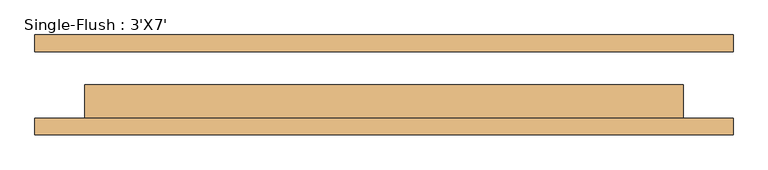
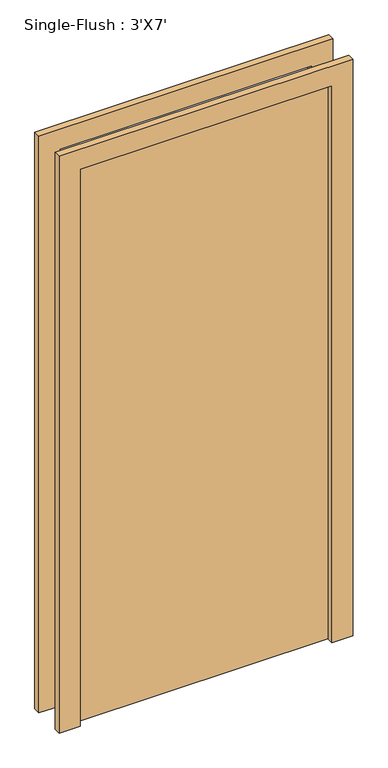
"""IFC4 building model written with IfcOpenShell, lengths in millimetres: door geometry, Single-Flush : 3'X7'."""

from ifc_helpers import new_model, si_unit, frame, origin, origin_with_axes, place, context, project, spatial, polyline, outline, extrude, source, transform, mapped, element, save


def single_flush_3_x7_310a3c6c(model_context):
    return source(origin(), model_context, "Body", "SweptSolid", [
        extrude(outline(polyline([(2209.8, -533.4), (0.0, -533.4), (0.0, -457.2), (2133.6, -457.2), (2133.6, 457.2), (0.0, 457.2), (0.0, 533.4), (2209.8, 533.4), (2209.8, -533.4)])), frame((0.0, -76.2, 0.0), z_axis=(0.0, 1.0, 0.0), x_axis=(0.0, 0.0, 1.0)), (0.0, 0.0, 1.0), 25.4),
        extrude(outline(polyline([(2209.8, 533.4), (2209.8, -533.4), (0.0, -533.4), (0.0, -457.2), (2133.6, -457.2), (2133.6, 457.2), (0.0, 457.2), (0.0, 533.4), (2209.8, 533.4)])), frame((0.0, 50.8, 0.0), z_axis=(0.0, 1.0, 0.0), x_axis=(0.0, 0.0, 1.0)), (0.0, 0.0, 1.0), 25.4),
        extrude(outline(polyline([(457.2, 0.0), (457.2, -50.8), (-457.2, -50.8), (-457.2, 0.0), (457.2, 0.0)])), origin_with_axes(), (0.0, 0.0, 1.0), 2133.6),
    ])


if __name__ == "__main__":
    model = new_model("IFC4")
    model_context = context("Model", 3, world=origin())
    ifc_project = project(units=[si_unit("LENGTHUNIT", "METRE", prefix="MILLI")], contexts=[model_context])
    site = spatial("IfcSite", under=ifc_project)
    building = spatial("IfcBuilding", under=site)
    placement = place(None, origin())
    single_flush_3_x7_shape = single_flush_3_x7_310a3c6c(model_context)
    element("IfcDoor", 1, ObjectType="Single-Flush : 3'X7'", at=placement, inside=building, context=model_context, shape_type="MappedRepresentation", body=[
        mapped(single_flush_3_x7_shape, transform((0.0, 0.0, 0.0), x_axis=(1.0, 0.0, 0.0), y_axis=(0.0, 1.0, 0.0), z_axis=(0.0, 0.0, 1.0))),
    ])
    save(model, "model.ifc")

# Revit data of these elements
# Type "Single-Flush : 3'X7'"
#   Type Mark = "8"
#   Construction Type Id = "MDOOR"
#   Assembly Code = "C1020"
#   Analytic Construction = "Metal"
#   Thickness = 0' - 2"
#   Heat Transfer Coefficient (U) = 0.651978 BTU/(h·ft²·°F)
#   Height = 7' - 0"
#   Trim Projection Ext = 0' - 1"
#   Trim Projection Int = 0' - 1"
#   Trim Width = 0' - 3"
#   Width = 3' - 0"
#   Define Thermal Properties by = 1
#   Door Material = Door - Panel
#   Frame Material = Door - Frame
#   Visual Light Transmittance = 0
#   Solar Heat Gain Coefficient = 0
#   Function = (empty or 0)
#   Wall Closure = (empty or 0)
# Element 1 (IfcDoor, "Single-Flush : 3'X7'")
#   Materials on its faces: "Door - Frame", "Door - Panel"
# Materials
#   "Door - Panel": class "Wood", colour RGB 210 159 95, transparency 0, Cost = 0
#   "Door - Frame": colour RGB 118 70 51, transparency 0, Cost = 0
